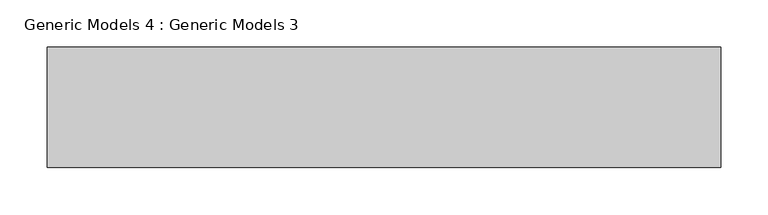
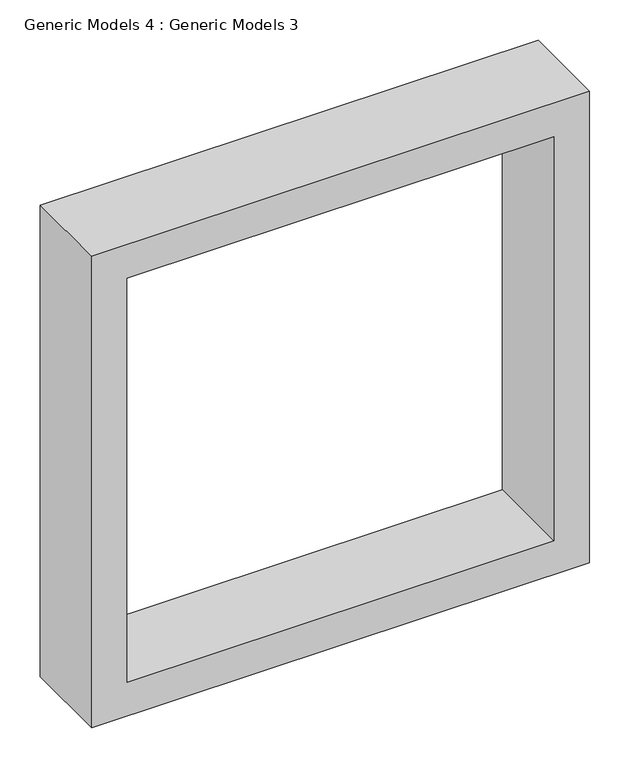
"""IFC4 building model written with IfcOpenShell, lengths in millimetres: proxy geometry, Generic Models 4 : Generic Models 3."""

from ifc_helpers import new_model, si_unit, frame, origin, place, context, project, spatial, polyline, outline, extrude, source, transform, mapped, element, save


def generic_models_4_generic_models_3_1a75a499(model_context):
    return source(origin(), model_context, "Body", "SweptSolid", [
        extrude(outline(polyline([(3098.8, -5721.373248), (3098.8, -6432.573248), (2387.6, -6432.573248), (2387.6, -5721.373248), (3098.8, -5721.373248)]), holes=[polyline([(3048.0, -5772.173248), (2438.4, -5772.173248), (2438.4, -6381.773248), (3048.0, -6381.773248), (3048.0, -5772.173248)])]), frame((0.0, -3899.4866303, 0.0), z_axis=(0.0, 1.0, 0.0), x_axis=(0.0, 0.0, 1.0)), (0.0, 0.0, 1.0), 127.0),
    ])


if __name__ == "__main__":
    model = new_model("IFC4")
    model_context = context("Model", 3, world=origin())
    ifc_project = project(units=[si_unit("LENGTHUNIT", "METRE", prefix="MILLI")], contexts=[model_context])
    site = spatial("IfcSite", under=ifc_project)
    building = spatial("IfcBuilding", under=site)
    placement = place(None, origin())
    generic_models_4_generic_models_3_shape = generic_models_4_generic_models_3_1a75a499(model_context)
    element("IfcBuildingElementProxy", 1, Name="Generic Models 4 : Generic Models 3", ObjectType="Generic Models 4 : Generic Models 3", at=placement, inside=building, context=model_context, shape_type="MappedRepresentation", body=[
        mapped(generic_models_4_generic_models_3_shape, transform((0.0, 0.0, 0.0), x_axis=(1.0, 0.0, 0.0), y_axis=(0.0, 1.0, 0.0), z_axis=(0.0, 0.0, 1.0))),
    ])
    save(model, "model.ifc")

# Revit data of these elements
# Element 1 (IfcBuildingElementProxy, "Generic Models 4 : Generic Models 3")
#   Materials on its faces: "BLACK FRAMING 6\""
# Materials
#   "BLACK FRAMING 6\"": class "Generic", colour RGB 120 120 120, transparency 0, Cost = 0
